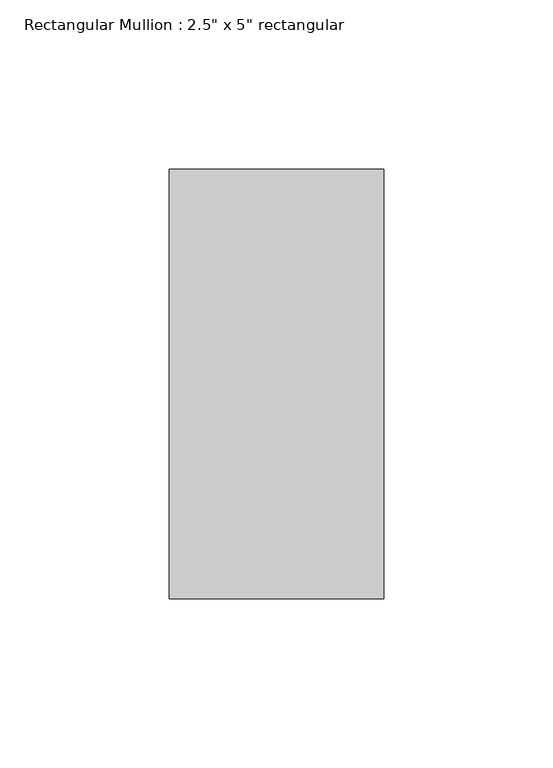
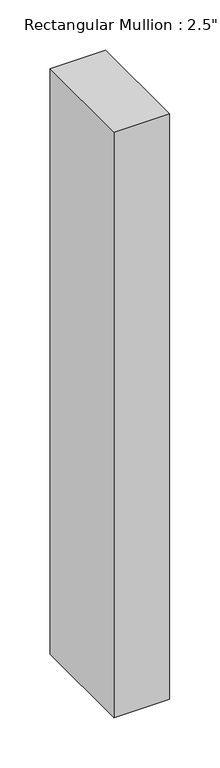
"""IFC4 building model written with IfcOpenShell, lengths in millimetres: member geometry."""

from ifc_helpers import new_model, si_unit, frame, origin, place, context, project, spatial, polyline, outline, extrude, source, transform, mapped, element, save


def member_e606956e(model_context):
    return source(origin(), model_context, "Body", "SweptSolid", [
        extrude(outline(polyline([(0.0, 63.5), (0.0, -63.5), (-63.5, -63.5), (-63.5, 63.5), (0.0, 63.5)])), frame((0.0, 0.0, -709.0542001), z_axis=(0.0, 0.0, 1.0), x_axis=(1.0, 0.0, 0.0)), (0.0, 0.0, 1.0), 709.0542001),
    ])


if __name__ == "__main__":
    model = new_model("IFC4")
    model_context = context("Model", 3, world=origin())
    ifc_project = project(units=[si_unit("LENGTHUNIT", "METRE", prefix="MILLI")], contexts=[model_context])
    site = spatial("IfcSite", under=ifc_project)
    building = spatial("IfcBuilding", under=site)
    placement = place(None, origin())
    member_shape = member_e606956e(model_context)
    element("IfcMember", 1, ObjectType="Rectangular Mullion : 2.5\" x 5\" rectangular", at=placement, inside=building, context=model_context, shape_type="MappedRepresentation", body=[
        mapped(member_shape, transform((0.0, 0.0, 0.0), x_axis=(1.0, 0.0, 0.0), y_axis=(0.0, 1.0, 0.0), z_axis=(0.0, 0.0, 1.0))),
    ])
    save(model, "model.ifc")

# Revit data of these elements
# Type "Rectangular Mullion : 2.5\" x 5\" rectangular"
#   built-in parameter 1007304 = 0.416667 (stored number, unit not read)
#   built-in parameter 1007301 = 0.104167 (stored number, unit not read)
#   built-in parameter 1007300 = 0.104167 (stored number, unit not read)
# Element 1 (IfcMember, "Rectangular Mullion : 2.5\" x 5\" rectangular")
#   Materials on its faces: "Aluminum"
# Materials
#   "Aluminum": class "Metal", colour RGB 247 247 247, transparency 0, Description = "Aluminum 6061", Cost = 0
